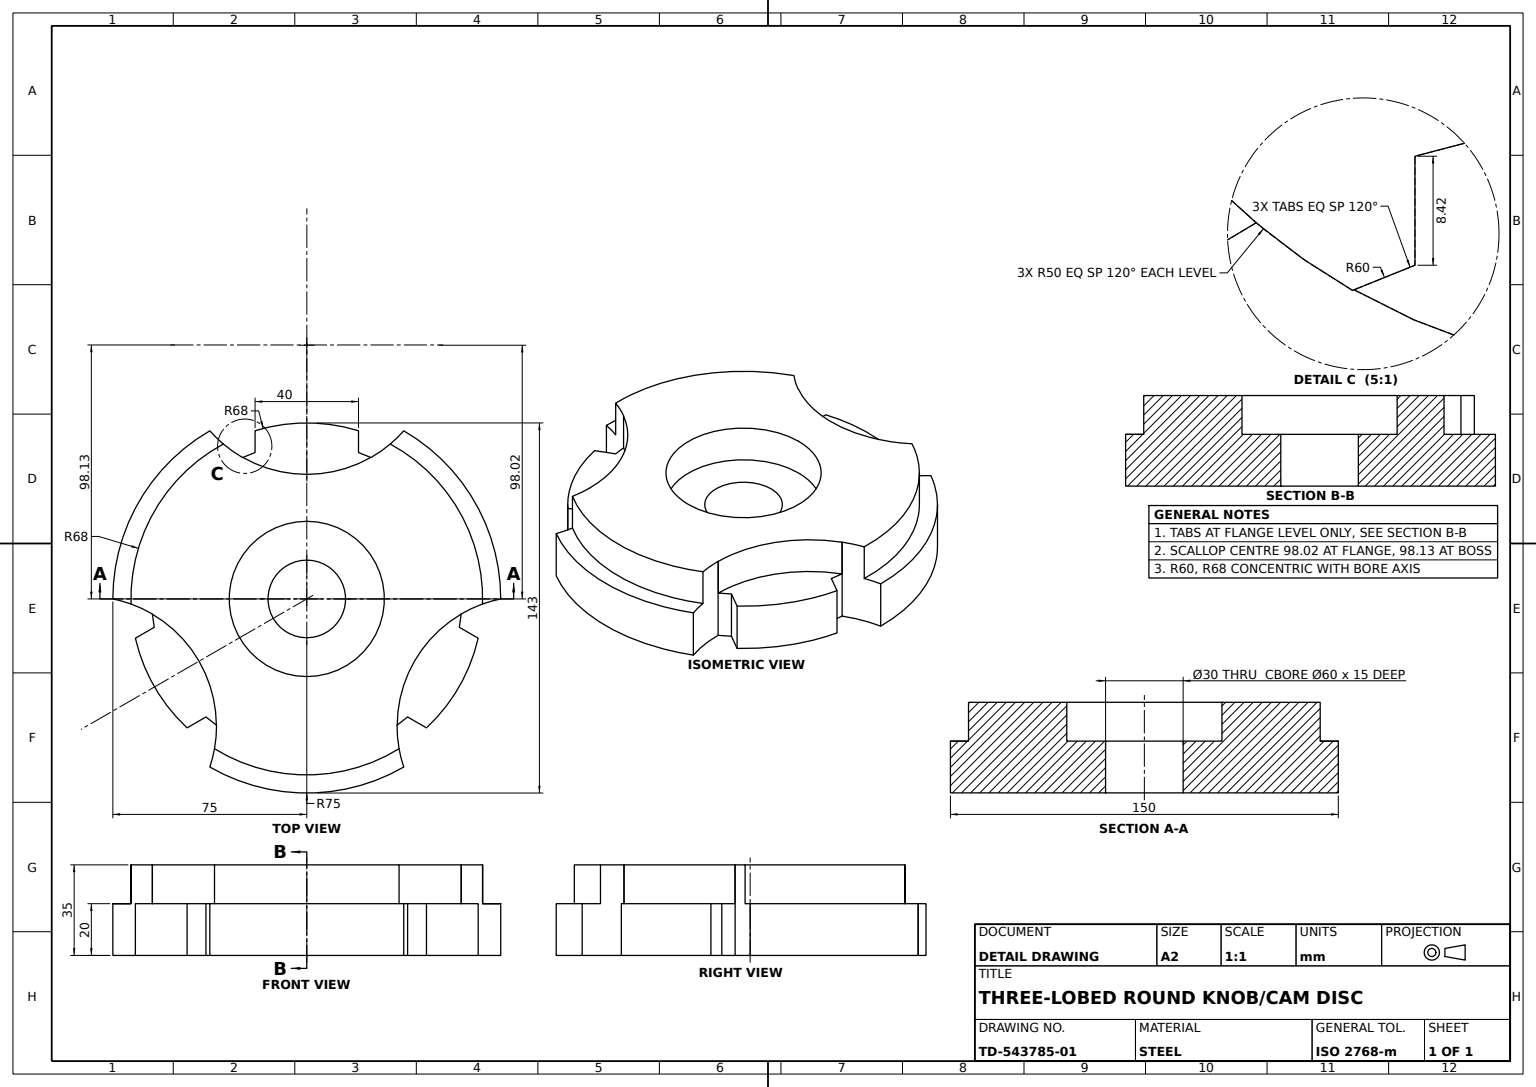
from build123d import *

# Parameters (mm, degrees)
LOBED_BASE_20MM_DEPTH          = 20
NOTCHED_START                  = -20
NOTCHED_STEP_BOSS_20MM_DEPTH   = 20
LOBED_TOP_STEP_BOSS_15MM_DEPTH = 15
COUNTERBORE_PROFILE_60_R       = 30
COUNTERBORE_60X15_DEPTH        = 15
CENTER_BORE_PROFILE_30_R       = 15
CENTER_BORE_30_DEPTH           = 60


with BuildPart() as part:
    # Lobed Base Profile → Lobed Base 20mm (new body)
    with BuildSketch(Plane(origin=(0, 0, 0), x_dir=(1, 0, 0), z_dir=(0, 1, 0))):
        with BuildLine():
            ThreePointArc((-37.5, 64.951905284), (-64.951905284, 37.5), (-75, 0))
            ThreePointArc((-75, 0), (-41.589827904, -24.011898336), (-37.5, -64.951905284))
            ThreePointArc((-37.5, -64.951905284), (0, -75), (37.5, -64.951905284))
            ThreePointArc((37.5, -64.951905284), (41.589827904, -24.011898336), (75, 0))
            ThreePointArc((75, 0), (64.951905284, 37.5), (37.5, 64.951905284))
            ThreePointArc((37.5, 64.951905284), (0, 48.023796672), (-37.5, 64.951905284))
        make_face()
    extrude(amount=LOBED_BASE_20MM_DEPTH)

    # Notched Step Profile → Notched Step Boss 20mm (add)
    with BuildSketch(Plane(origin=(0, 20, 0), x_dir=(1, 0, 0), z_dir=(0, 1, 0)).offset(NOTCHED_START)):
        with BuildLine():
            Line((66.284989118, -15.175645543), (58.989794856, -10.963763172))
            ThreePointArc((58.989794856, -10.963763172), (59.409752684, -8.395313338), (59.717932727, -5.811067957))
            ThreePointArc((59.717932727, -5.811067957), (41.589827904, -24.011898336), (34.891498837, -48.811712825))
            ThreePointArc((34.891498837, -48.811712825), (36.975430965, -47.252698388), (38.989794856, -45.604779323))
            Line((38.989794856, -45.604779323), (46.284989118, -49.816661694))
            ThreePointArc((46.284989118, -49.816661694), (58.889727457, -34), (66.284989118, -15.175645543))
        make_face()
        with BuildLine():
            Line((20, 64.992307237), (20, 56.568542495))
            ThreePointArc((20, 56.568542495), (22.434321719, 55.648011726), (24.82643389, 54.622780782))
            ThreePointArc((24.82643389, 54.622780782), (0, 48.023796672), (-24.82643389, 54.622780782))
            ThreePointArc((-24.82643389, 54.622780782), (-22.434321719, 55.648011726), (-20, 56.568542495))
            Line((-20, 56.568542495), (-20, 64.992307237))
            ThreePointArc((-20, 64.992307237), (0, 68), (20, 64.992307237))
        make_face()
        with BuildLine():
            Line((-46.284989118, -49.816661694), (-38.989794856, -45.604779323))
            ThreePointArc((-38.989794856, -45.604779323), (-36.975430965, -47.252698388), (-34.891498837, -48.811712825))
            ThreePointArc((-34.891498837, -48.811712825), (-41.589827904, -24.011898336), (-59.717932727, -5.811067957))
            ThreePointArc((-59.717932727, -5.811067957), (-59.409752684, -8.395313338), (-58.989794856, -10.963763172))
            Line((-58.989794856, -10.963763172), (-66.284989118, -15.175645543))
            ThreePointArc((-66.284989118, -15.175645543), (-58.889727457, -34), (-46.284989118, -49.816661694))
        make_face()
    extrude(amount=NOTCHED_STEP_BOSS_20MM_DEPTH)

    # Lobed Top Step Profile → Lobed Top Step Boss 15mm (add)
    with BuildSketch(Plane(origin=(0, 20, 0), x_dir=(1, 0, 0), z_dir=(0, 1, 0))):
        with BuildLine():
            ThreePointArc((-35.684614564, -57.884439044), (-34.845932731, -58.393158607), (-34, -58.889727457))
            ThreePointArc((-34, -58.889727457), (0, -68), (34, -58.889727457))
            ThreePointArc((34, -58.889727457), (34.845932731, -58.393158607), (35.684614564, -57.884439044))
            ThreePointArc((35.684614564, -57.884439044), (35.081055876, -53.366171445), (34.891498837, -48.811712825))
            ThreePointArc((34.891498837, -48.811712825), (34.925233252, -48.78758123), (34.958950977, -48.763426321))
            ThreePointArc((34.958950977, -48.763426321), (41.65016617, -24.031498852), (59.713066847, -5.860857251))
            ThreePointArc((59.713066847, -5.860857251), (59.715504976, -5.835963111), (59.717932727, -5.811067957))
            ThreePointArc((59.717932727, -5.811067957), (63.756988112, -3.697999858), (67.971701978, -1.961563214))
            ThreePointArc((67.971701978, -1.961563214), (67.992925126, -0.98088366), (68, 0))
            ThreePointArc((68, 0), (58.393158607, 34.845932731), (32.287087414, 59.846002258))
            ThreePointArc((32.287087414, 59.846002258), (28.675932236, 57.064171303), (24.82643389, 54.622780782))
            ThreePointArc((24.82643389, 54.622780782), (24.782049597, 54.642932002), (24.737648948, 54.663047157))
            ThreePointArc((24.737648948, 54.663047157), (0.01107673, 48.127580971), (-24.712484549, 54.674428277))
            ThreePointArc((-24.712484549, 54.674428277), (-24.769472681, 54.648634229), (-24.82643389, 54.622780782))
            ThreePointArc((-24.82643389, 54.622780782), (-28.675932236, 57.064171303), (-32.287087414, 59.846002258))
            ThreePointArc((-32.287087414, 59.846002258), (-58.889727457, 34), (-67.971701978, -1.961563214))
            ThreePointArc((-67.971701978, -1.961563214), (-63.756988112, -3.697999858), (-59.717932727, -5.811067957))
            ThreePointArc((-59.717932727, -5.811067957), (-59.713515872, -5.856280575), (-59.709064787, -5.901489836))
            ThreePointArc((-59.709064787, -5.901489836), (-41.66322938, -24.054276698), (-34.965372512, -48.758822023))
            ThreePointArc((-34.965372512, -48.758822023), (-34.928445686, -48.785281407), (-34.891498837, -48.811712825))
            ThreePointArc((-34.891498837, -48.811712825), (-35.081055876, -53.366171445), (-35.684614564, -57.884439044))
        make_face()
    extrude(amount=LOBED_TOP_STEP_BOSS_15MM_DEPTH)

    # Counterbore Profile Ø60 → Counterbore Ø60x15 (cut)
    with BuildSketch(Plane(origin=(0, 35, 0), x_dir=(1, 0, 0), z_dir=(0, 1, 0))):
        with Locations(Location((0, 0, 0), (0, 0, 270))):
            Circle(COUNTERBORE_PROFILE_60_R)
    extrude(amount=-COUNTERBORE_60X15_DEPTH, mode=Mode.SUBTRACT)

    # Center Bore Profile Ø30 → Center Bore Ø30 (cut)
    with BuildSketch(Plane(origin=(0, 20, 0), x_dir=(1, 0, 0), z_dir=(0, 1, 0))):
        with Locations(Location((0, 0, 0), (0, 0, 270))):
            Circle(CENTER_BORE_PROFILE_30_R)
    extrude(amount=-CENTER_BORE_30_DEPTH, mode=Mode.SUBTRACT)


solid = part.part
